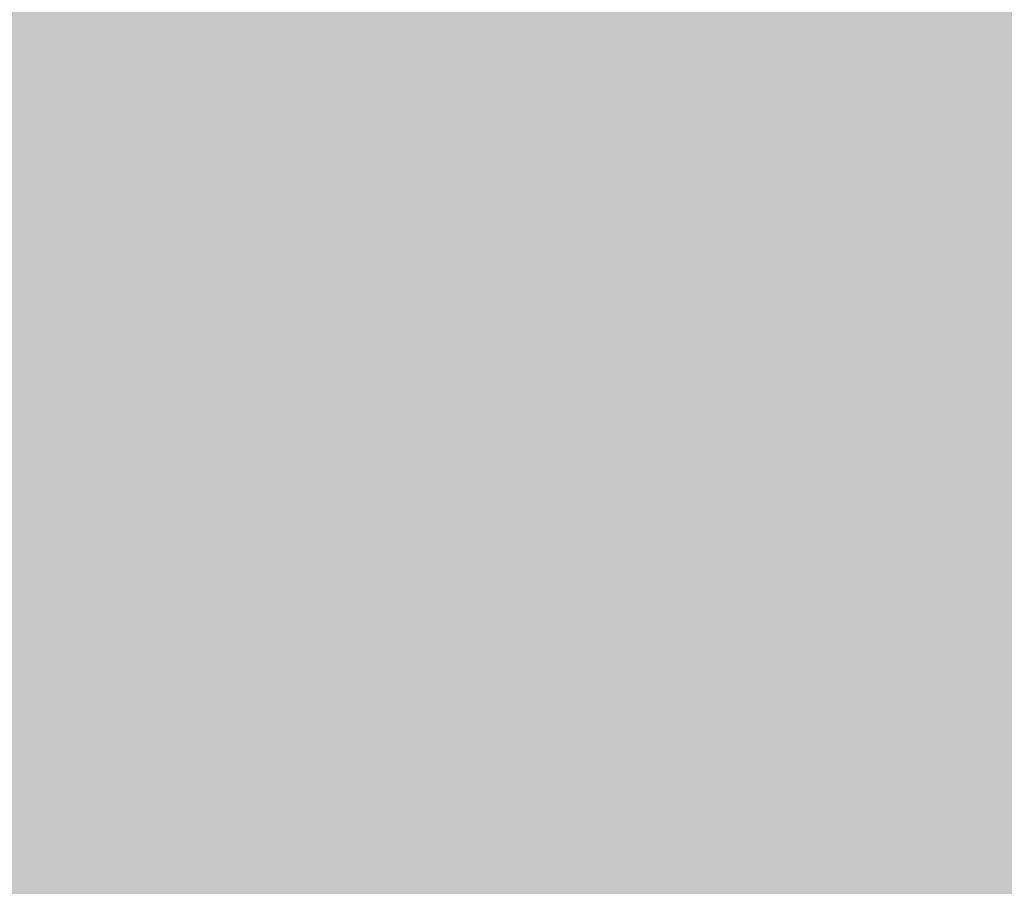
# Model space of a CAD drawing. Units: feet. Extents: x 3168 to 4724, y 827 to 1477.
# Tile 37 of 256: x 3270.27 to 3284.48, y 1074.89 to 1087.4. Entities that reach past the tile are written whole.
import ezdxf

# ---------------------------------------------------------------- set-up
doc = ezdxf.new("R2010")
doc.units = ezdxf.units.FT
doc.layers.add('A-ELEV-PATT', color=8, linetype='Continuous', lineweight=13)

msp = doc.modelspace()

# ---------------------------------------------------------------- hatches: boundary and pattern name
at = {"layer": 'A-ELEV-PATT'}
h = msp.add_hatch(color=256, dxfattribs=at)
h.dxf.hatch_style = 1
edge = h.paths.add_edge_path()
edge.add_ellipse((3552.906, 979.22), major_axis=(36.745, 0), ratio=0.484848, start_angle=0, end_angle=360)
edge = h.paths.add_edge_path()
edge.add_ellipse((3559.892, 929.252), major_axis=(36.745, 0), ratio=0.484848, start_angle=0, end_angle=360)
edge = h.paths.add_edge_path()
edge.add_line((3299.317, 1198.606), (3479.917, 1198.606))
edge.add_line((3479.917, 1198.606), (3479.917, 1209.869))
edge.add_spline(control_points=[(3479.917, 1209.869), (3464.301, 1209.869), (3448.686, 1209.869), (3410.949, 1209.869), (3388.828, 1209.869), (3355.647, 1209.869), (3344.586, 1209.869), (3327.996, 1209.869), (3322.466, 1209.869), (3314.17, 1209.869), (3311.405, 1209.869), (3307.257, 1209.869), (3305.875, 1209.869), (3303.801, 1209.869), (3303.11, 1209.869), (3302.073, 1209.869), (3301.727, 1209.869), (3301.209, 1209.869), (3301.036, 1209.869), (3300.777, 1209.869), (3300.69, 1209.869), (3300.561, 1209.869), (3300.517, 1209.869), (3300.453, 1209.869), (3300.431, 1209.869), (3300.399, 1209.869), (3300.388, 1209.869), (3300.366, 1209.869), (3300.346, 1209.869), (3300.346, 1209.869), (3300.346, 1209.869), (3300.343, 1209.869), (3300.341, 1209.869), (3300.338, 1209.869), (3300.337, 1209.869), (3300.334, 1209.869), (3300.332, 1209.869), (3300.326, 1209.869), (3300.321, 1209.869), (3300.311, 1209.869), (3300.306, 1209.869), (3300.291, 1209.869), (3300.28, 1209.869), (3300.232, 1209.869), (3300.195, 1209.869), (3299.951, 1209.871), (3299.745, 1209.874), (3299.437, 1209.883), (3299.334, 1209.887), (3299.181, 1209.893), (3299.13, 1209.895), (3298.652, 1209.917), (3298.229, 1209.946), (3297.602, 1210.002), (3297.393, 1210.023), (3297.083, 1210.058), (3296.979, 1210.07), (3296.293, 1210.155), (3295.718, 1210.243), (3294.869, 1210.399), (3294.588, 1210.454), (3294.169, 1210.543), (3294.03, 1210.574), (3291.707, 1211.101), (3289.654, 1211.813), (3285.776, 1213.564), (3283.951, 1214.603), (3280.512, 1216.98), (3278.897, 1218.318), (3276.38, 1220.829), (3275.416, 1221.918), (3274.039, 1223.708), (3273.581, 1224.35), (3273.143, 1225.016)], knot_values=[39.119033, 39.119033, 39.119033, 39.119033, 39.286353, 39.286353, 39.523379, 39.523379, 39.641892, 39.641892, 39.701148, 39.701148, 39.730777, 39.730777, 39.745591, 39.745591, 39.752998, 39.752998, 39.756701, 39.756701, 39.758553, 39.758553, 39.759479, 39.759479, 39.759942, 39.759942, 39.760173, 39.760173, 39.760289, 39.760289, 39.760405, 39.760405, 39.760463, 39.760463, 39.763389, 39.763389, 39.764851, 39.764851, 39.767304, 39.767304, 39.773825, 39.773825, 39.78057, 39.78057, 39.79477, 39.79477, 39.845194, 39.845194, 40.126715, 40.126715, 40.267476, 40.267476, 40.337856, 40.337856, 40.927023, 40.927023, 41.221606, 41.221606, 41.368898, 41.368898, 42.202622, 42.202622, 42.619485, 42.619485, 42.827916, 42.827916, 46.118323, 46.118323, 49.408731, 49.408731, 52.699139, 52.699139, 54.927489, 54.927489, 56.104228, 56.104228, 56.104228, 56.104228], weights=[1, 1, 1, 1, 1, 1, 1, 1, 1, 1, 1, 1, 1, 1, 1, 1, 1, 1, 1, 1, 1, 1, 1, 1, 1, 1, 1, 1, 1, 1, 1, 1, 1, 1, 1, 1, 1, 1, 1, 1, 1, 1, 1, 1, 1, 1, 1, 1, 1, 1, 1, 1, 1, 1, 1, 1, 1, 1, 1, 1, 1, 1, 1, 1, 1, 1, 1, 1, 1, 1, 1, 1, 1, 1], degree=3, periodic=0)
edge.add_line((3273.143, 1225.016), (3273.143, 1099.016))
edge.add_line((3273.143, 1099.016), (3299.317, 1099.016))
edge.add_line((3299.317, 1099.016), (3299.317, 1198.606))
edge = h.paths.add_edge_path()
edge.add_line((3304.758, 1324.158), (3479.917, 1324.158))
edge.add_line((3479.917, 1324.158), (3479.917, 1335.715))
edge.add_line((3479.917, 1335.715), (3269.162, 1335.715))
edge.add_spline(control_points=[(3269.162, 1335.715), (3264.024, 1335.715), (3258.364, 1328.958), (3259.264, 1323.9)], knot_values=[0, 0, 0, 0, 15.412191, 15.412191, 15.412191, 15.412191], degree=3, periodic=0)
edge.add_line((3259.264, 1323.9), (3265.517, 1288.769))
edge.add_line((3265.517, 1288.769), (3275.265, 1261.546))
edge.add_line((3275.265, 1261.546), (3304.758, 1261.546))
edge.add_line((3304.758, 1261.546), (3304.758, 1324.158))
h = msp.add_hatch(color=256, dxfattribs=at)
h.dxf.hatch_style = 1
h.paths.add_polyline_path([(3384.525, 1099.016), (3335.029, 1099.016), (3299.317, 1099.016), (3273.143, 1099.016), (3217.565, 1099.016), (3168.069, 827.116), (3335.029, 827.116)])

doc.saveas('drawing.dxf')
